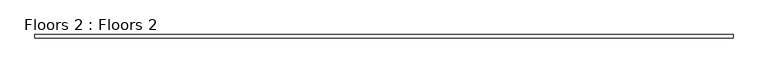
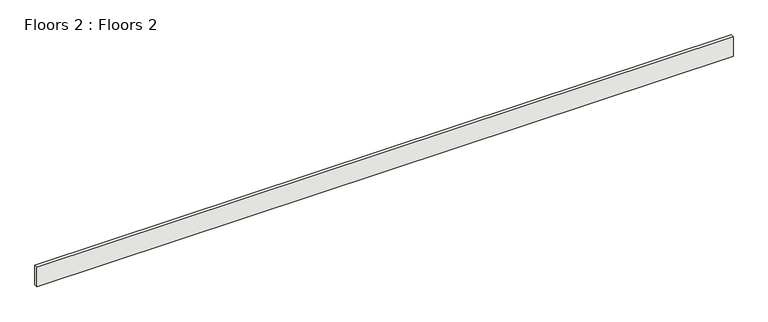
"""IFC4 building model written with IfcOpenShell, lengths in millimetres: slab geometry, Floors 2 : Floors 2."""

from ifc_helpers import new_model, si_unit, origin, origin_with_axes, place, context, project, spatial, polyline, outline, extrude, source, transform, mapped, element, save


def floors_2_floors_2_9b529a88(model_context):
    return source(origin(), model_context, "Body", "SweptSolid", [
        extrude(outline(polyline([(3889.1430349, 400.7055142), (-6524.8569651, 400.7055142), (-6524.8569651, 451.5055142), (3889.1430349, 451.5055142), (3889.1430349, 400.7055142)])), origin_with_axes(), (0.0, 0.0, 1.0), 304.8),
    ])


if __name__ == "__main__":
    model = new_model("IFC4")
    model_context = context("Model", 3, world=origin())
    ifc_project = project(units=[si_unit("LENGTHUNIT", "METRE", prefix="MILLI")], contexts=[model_context])
    site = spatial("IfcSite", under=ifc_project)
    building = spatial("IfcBuilding", under=site)
    placement = place(None, origin())
    floors_2_floors_2_shape = floors_2_floors_2_9b529a88(model_context)
    element("IfcSlab", 1, ObjectType="Floors 2 : Floors 2", at=placement, inside=building, context=model_context, shape_type="MappedRepresentation", body=[
        mapped(floors_2_floors_2_shape, transform((0.0, 0.0, 0.0), x_axis=(1.0, 0.0, 0.0), y_axis=(0.0, 1.0, 0.0), z_axis=(0.0, 0.0, 1.0))),
    ])
    save(model, "model.ifc")

# Revit data of these elements
# Element 1 (IfcSlab, "Floors 2 : Floors 2")
#   Materials on its faces: "1 wall brown", "Default Floor"
# Materials
#   "1 wall brown": class "Generic", colour RGB 61 46 37, transparency 0, Cost = 0
#   "Default Floor": colour RGB 128 128 128, transparency 0, Cost = 0
